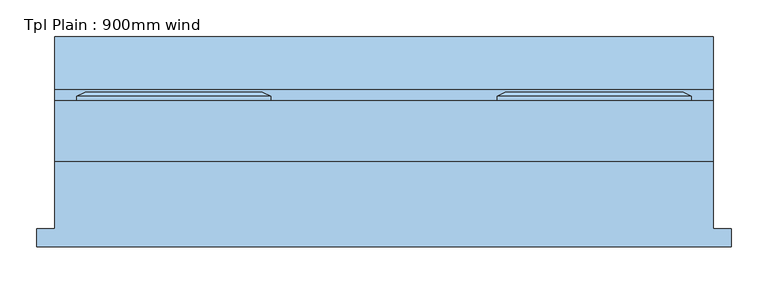
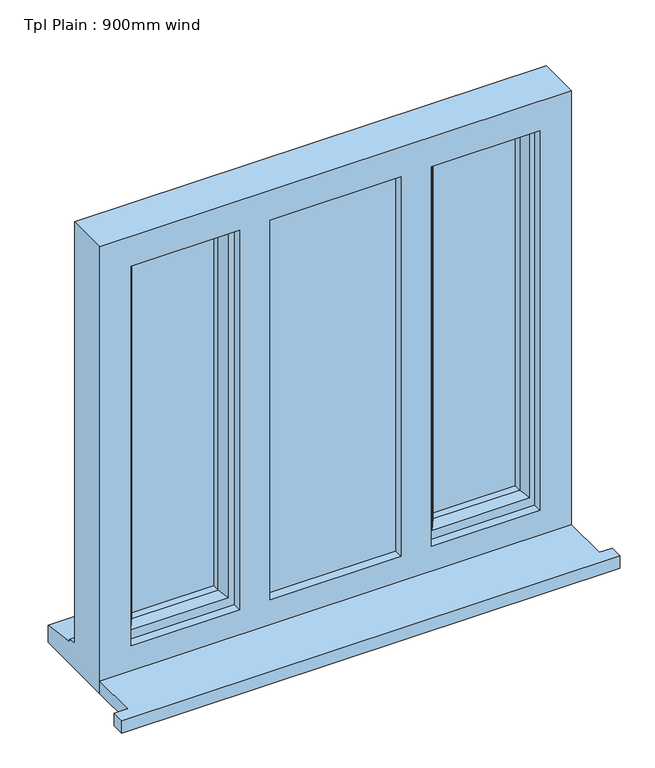
"""IFC4 building model written with IfcOpenShell, lengths in millimetres: window geometry, Tpl Plain : 900mm wind."""

from ifc_helpers import new_model, si_unit, frame, origin, place, context, project, spatial, polyline, outline, extrude, faceted_brep, source, transform, mapped, element, save


def tpl_plain_900mm_wind_8db11632(model_context):
    return source(origin(), model_context, "Body", "SolidModel", [
        extrude(outline(polyline([(-900.0, -129.0434322), (-900.0, -104.0434322), (-875.0, -104.0434322), (-875.0, -12.0434322), (25.0, -12.0434322), (25.0, -104.0434322), (50.0, -104.0434322), (50.0, -129.0434322), (-900.0, -129.0434322)])), frame((0.0, 0.0, 1500.0), z_axis=(0.0, 0.0, 1.0), x_axis=(1.0, 0.0, 0.0)), (0.0, 0.0, 1.0), 25.0),
        faceted_brep([(-270.0, 70.9565678, 2370.0), (-270.0, 76.7300705, 2370.0), (-270.0, 76.7300705, 1553.0), (-270.0, 70.9565678, 1553.0), (-260.0, 5.9565678, 2360.0), (-260.0, 70.9565678, 2360.0), (-260.0, 70.9565678, 1563.0), (-260.0, 5.9565678, 1563.0), (-220.0, 20.4494677, 2320.0), (-230.1480377, 5.9565678, 2330.1480377), (-230.1480377, 5.9565678, 1592.8519623), (-220.0, 20.4494677, 1603.0), (-220.0, 34.9565678, 2320.0), (-220.0, 34.9565678, 1603.0), (-230.0, 58.9565678, 2330.0), (-230.0, 34.9565678, 2330.0), (-230.0, 34.9565678, 1593.0), (-230.0, 58.9565678, 1593.0), (-220.0, 76.7300705, 2320.0), (-220.0, 58.9565678, 2320.0), (-220.0, 58.9565678, 1603.0), (-220.0, 76.7300705, 1603.0), (-237.4457548, 82.5035732, 2337.4457548), (-237.4457548, 82.5035732, 1585.5542452), (-259.2153903, 82.5035732, 2359.2153903), (-259.2153903, 82.5035732, 1563.7846097), (-5.0, 76.7300705, 1553.0), (-5.0, 70.9565678, 1553.0), (-15.0, 70.9565678, 1563.0), (-15.0, 5.9565678, 1563.0), (-44.8519623, 5.9565678, 1592.8519623), (-55.0, 20.4494677, 1603.0), (-55.0, 34.9565678, 1603.0), (-45.0, 34.9565678, 1593.0), (-45.0, 58.9565678, 1593.0), (-55.0, 58.9565678, 1603.0), (-55.0, 76.7300705, 1603.0), (-37.5542452, 82.5035732, 1585.5542452), (-15.7846097, 82.5035732, 1563.7846097), (-5.0, 76.7300705, 2370.0), (-5.0, 70.9565678, 2370.0), (-15.0, 70.9565678, 2360.0), (-15.0, 5.9565678, 2360.0), (-44.8519623, 5.9565678, 2330.1480377), (-55.0, 20.4494677, 2320.0), (-55.0, 34.9565678, 2320.0), (-45.0, 34.9565678, 2330.0), (-45.0, 58.9565678, 2330.0), (-55.0, 58.9565678, 2320.0), (-55.0, 76.7300705, 2320.0), (-37.5542452, 82.5035732, 2337.4457548), (-15.7846097, 82.5035732, 2359.2153903)], [[[0, 1, 2, 3]], [[4, 5, 6, 7]], [[8, 9, 10, 11]], [[12, 8, 11, 13]], [[14, 15, 16, 17]], [[18, 19, 20, 21]], [[22, 18, 21, 23]], [[1, 24, 25, 2]], [[3, 2, 26, 27]], [[7, 6, 28, 29]], [[11, 10, 30, 31]], [[13, 11, 31, 32]], [[17, 16, 33, 34]], [[21, 20, 35, 36]], [[23, 21, 36, 37]], [[2, 25, 38, 26]], [[27, 26, 39, 40]], [[29, 28, 41, 42]], [[31, 30, 43, 44]], [[32, 31, 44, 45]], [[34, 33, 46, 47]], [[36, 35, 48, 49]], [[37, 36, 49, 50]], [[26, 38, 51, 39]], [[40, 39, 1, 0]], [[3, 27, 40, 0], [5, 41, 28, 6]], [[42, 41, 5, 4]], [[7, 29, 42, 4], [9, 43, 30, 10]], [[44, 43, 9, 8]], [[45, 44, 8, 12]], [[15, 46, 33, 16], [13, 32, 45, 12]], [[47, 46, 15, 14]], [[17, 34, 47, 14], [19, 48, 35, 20]], [[49, 48, 19, 18]], [[50, 49, 18, 22]], [[24, 51, 38, 25], [23, 37, 50, 22]], [[39, 51, 24, 1]]]),
        faceted_brep([(-580.0, 70.9565678, 2370.0), (-580.0, 76.7300705, 2370.0), (-845.0, 76.7300705, 2370.0), (-845.0, 70.9565678, 2370.0), (-590.0, 5.9565678, 2360.0), (-590.0, 70.9565678, 2360.0), (-835.0, 70.9565678, 2360.0), (-835.0, 5.9565678, 2360.0), (-630.0, 20.4494677, 2320.0), (-619.8519623, 5.9565678, 2330.1480377), (-805.1480377, 5.9565678, 2330.1480377), (-795.0, 20.4494677, 2320.0), (-630.0, 34.9565678, 2320.0), (-795.0, 34.9565678, 2320.0), (-620.0, 58.9565678, 2330.0), (-620.0, 34.9565678, 2330.0), (-805.0, 34.9565678, 2330.0), (-805.0, 58.9565678, 2330.0), (-630.0, 76.7300705, 2320.0), (-630.0, 58.9565678, 2320.0), (-795.0, 58.9565678, 2320.0), (-795.0, 76.7300705, 2320.0), (-611.1854344, 82.5035732, 2338.8145656), (-813.8145656, 82.5035732, 2338.8145656), (-591.6307806, 82.5035732, 2358.3692194), (-833.3692194, 82.5035732, 2358.3692194), (-845.0, 76.7300705, 1553.0), (-845.0, 70.9565678, 1553.0), (-835.0, 70.9565678, 1563.0), (-835.0, 5.9565678, 1563.0), (-805.1480377, 5.9565678, 1592.8519623), (-795.0, 20.4494677, 1603.0), (-795.0, 34.9565678, 1603.0), (-805.0, 34.9565678, 1593.0), (-805.0, 58.9565678, 1593.0), (-795.0, 58.9565678, 1603.0), (-795.0, 76.7300705, 1603.0), (-813.8145656, 82.5035732, 1584.1854344), (-833.3692194, 82.5035732, 1564.6307806), (-580.0, 76.7300705, 1553.0), (-580.0, 70.9565678, 1553.0), (-590.0, 70.9565678, 1563.0), (-590.0, 5.9565678, 1563.0), (-619.8519623, 5.9565678, 1592.8519623), (-630.0, 20.4494677, 1603.0), (-630.0, 34.9565678, 1603.0), (-620.0, 34.9565678, 1593.0), (-620.0, 58.9565678, 1593.0), (-630.0, 58.9565678, 1603.0), (-630.0, 76.7300705, 1603.0), (-611.1854344, 82.5035732, 1584.1854344), (-591.6307806, 82.5035732, 1564.6307806)], [[[0, 1, 2, 3]], [[4, 5, 6, 7]], [[8, 9, 10, 11]], [[12, 8, 11, 13]], [[14, 15, 16, 17]], [[18, 19, 20, 21]], [[22, 18, 21, 23]], [[1, 24, 25, 2]], [[3, 2, 26, 27]], [[7, 6, 28, 29]], [[11, 10, 30, 31]], [[13, 11, 31, 32]], [[17, 16, 33, 34]], [[21, 20, 35, 36]], [[23, 21, 36, 37]], [[2, 25, 38, 26]], [[27, 26, 39, 40]], [[0, 3, 27, 40], [41, 28, 6, 5]], [[29, 28, 41, 42]], [[4, 7, 29, 42], [43, 30, 10, 9]], [[31, 30, 43, 44]], [[32, 31, 44, 45]], [[46, 33, 16, 15], [12, 13, 32, 45]], [[34, 33, 46, 47]], [[14, 17, 34, 47], [48, 35, 20, 19]], [[36, 35, 48, 49]], [[37, 36, 49, 50]], [[51, 38, 25, 24], [22, 23, 37, 50]], [[26, 38, 51, 39]], [[40, 39, 1, 0]], [[42, 41, 5, 4]], [[44, 43, 9, 8]], [[45, 44, 8, 12]], [[47, 46, 15, 14]], [[49, 48, 19, 18]], [[50, 49, 18, 22]], [[39, 51, 24, 1]]]),
        faceted_brep([(25.0, -12.0434322, 2400.0), (-875.0, -12.0434322, 2400.0), (-875.0, -12.0434322, 1500.0), (25.0, -12.0434322, 1500.0), (-35.0, -12.0434322, 2340.0), (-35.0, -12.0434322, 1575.0), (-242.0, -12.0434322, 1575.0), (-242.0, -12.0434322, 2340.0), (-300.0, -12.0434322, 2340.0), (-300.0, -12.0434322, 1575.0), (-550.0, -12.0434322, 1575.0), (-550.0, -12.0434322, 2340.0), (-608.0, -12.0434322, 2340.0), (-608.0, -12.0434322, 1575.0), (-815.0, -12.0434322, 1575.0), (-815.0, -12.0434322, 2340.0), (-875.0, 70.9565678, 2400.0), (-875.0, 70.9565678, 1551.0), (-875.0, 85.9565678, 1549.68767), (-875.0, 85.9565678, 1544.7449676), (-875.0, 158.4565678, 1533.8088847), (-875.0, 158.4565678, 1500.0), (25.0, 70.9565678, 2400.0), (25.0, 70.9565678, 1551.0), (-835.0, 70.9565678, 2360.0), (-835.0, 70.9565678, 1563.0), (-590.0, 70.9565678, 1563.0), (-590.0, 70.9565678, 2360.0), (-550.0, 70.9565678, 2360.0), (-550.0, 70.9565678, 1563.0), (-300.0, 70.9565678, 1563.0), (-300.0, 70.9565678, 2360.0), (-260.0, 70.9565678, 2360.0), (-260.0, 70.9565678, 1563.0), (-15.0, 70.9565678, 1563.0), (-15.0, 70.9565678, 2360.0), (-835.0, 5.9565678, 2360.0), (-835.0, 5.9565678, 1563.0), (-560.0, 5.9565678, 2360.0), (-290.0, 5.9565678, 2360.0), (-290.0, 5.9565678, 1563.0), (-560.0, 5.9565678, 1563.0), (-300.0, 5.9565678, 2340.0), (-550.0, 5.9565678, 2340.0), (-550.0, 5.9565678, 1575.0), (-300.0, 5.9565678, 1575.0), (-260.0, 5.9565678, 2360.0), (-15.0, 5.9565678, 2360.0), (-15.0, 5.9565678, 1563.0), (-260.0, 5.9565678, 1563.0), (-35.0, 5.9565678, 2340.0), (-242.0, 5.9565678, 2340.0), (-242.0, 5.9565678, 1575.0), (-35.0, 5.9565678, 1575.0), (-590.0, 5.9565678, 2360.0), (-590.0, 5.9565678, 1563.0), (-608.0, 5.9565678, 2340.0), (-815.0, 5.9565678, 2340.0), (-815.0, 5.9565678, 1575.0), (-608.0, 5.9565678, 1575.0), (-550.0, 29.9565678, 2360.0), (-300.0, 29.9565678, 2360.0), (-290.0, 29.9565678, 2360.0), (-560.0, 29.9565678, 2360.0), (25.0, 158.4565678, 1500.0), (25.0, 158.4565678, 1533.8088847), (25.0, 85.9565678, 1544.7449676), (25.0, 85.9565678, 1549.68767), (-550.0, 29.9565678, 1563.0), (-560.0, 29.9565678, 1563.0), (-290.0, 29.9565678, 1563.0), (-300.0, 29.9565678, 1563.0)], [[[0, 1, 2, 3], [4, 5, 6, 7], [8, 9, 10, 11], [12, 13, 14, 15]], [[2, 1, 16, 17, 18, 19, 20, 21]], [[17, 16, 22, 23], [24, 25, 26, 27], [28, 29, 30, 31], [32, 33, 34, 35]], [[25, 24, 36, 37]], [[38, 39, 40, 41], [42, 43, 44, 45]], [[46, 47, 48, 49], [50, 51, 52, 53]], [[36, 54, 55, 37], [56, 57, 58, 59]], [[57, 15, 14, 58]], [[1, 0, 22, 16]], [[36, 24, 27, 54]], [[35, 47, 46, 32]], [[60, 28, 31, 61, 62, 39, 38, 63]], [[15, 57, 56, 12]], [[50, 4, 7, 51]], [[11, 43, 42, 8]], [[23, 22, 0, 3, 64, 65, 66, 67]], [[35, 34, 48, 47]], [[4, 50, 53, 5]], [[43, 11, 10, 44]], [[12, 56, 59, 13]], [[27, 26, 55, 54]], [[29, 28, 60, 68]], [[68, 60, 63, 69]], [[69, 63, 38, 41]], [[62, 70, 40, 39]], [[70, 62, 61, 71]], [[71, 61, 31, 30]], [[33, 32, 46, 49]], [[51, 7, 6, 52]], [[8, 42, 45, 9]], [[64, 3, 2, 21]], [[65, 64, 21, 20]], [[66, 65, 20, 19]], [[67, 66, 19, 18]], [[23, 67, 18, 17]], [[26, 25, 37, 55]], [[34, 33, 49, 48]], [[41, 40, 70, 71, 30, 29, 68, 69]], [[6, 5, 53, 52]], [[45, 44, 10, 9]], [[59, 58, 14, 13]]]),
        extrude(outline(polyline([(-620.0, 34.9565678), (-805.0, 34.9565678), (-805.0, 58.9565678), (-620.0, 58.9565678), (-620.0, 34.9565678)])), frame((0.0, 0.0, 1593.0), z_axis=(0.0, 0.0, 1.0), x_axis=(1.0, 0.0, 0.0)), (0.0, 0.0, 1.0), 737.0),
        extrude(outline(polyline([(-560.0, 29.9565678), (-290.0, 29.9565678), (-290.0, 5.9565678), (-560.0, 5.9565678), (-560.0, 29.9565678)])), frame((0.0, 0.0, 1563.0), z_axis=(0.0, 0.0, 1.0), x_axis=(1.0, 0.0, 0.0)), (0.0, 0.0, 1.0), 797.0),
        extrude(outline(polyline([(-45.0, 34.9565678), (-230.0, 34.9565678), (-230.0, 58.9565678), (-45.0, 58.9565678), (-45.0, 34.9565678)])), frame((0.0, 0.0, 1593.0), z_axis=(0.0, 0.0, 1.0), x_axis=(1.0, 0.0, 0.0)), (0.0, 0.0, 1.0), 737.0),
    ])


if __name__ == "__main__":
    model = new_model("IFC4")
    model_context = context("Model", 3, world=origin())
    ifc_project = project(units=[si_unit("LENGTHUNIT", "METRE", prefix="MILLI")], contexts=[model_context])
    site = spatial("IfcSite", under=ifc_project)
    building = spatial("IfcBuilding", under=site)
    placement = place(None, origin())
    tpl_plain_900mm_wind_shape = tpl_plain_900mm_wind_8db11632(model_context)
    element("IfcWindow", 1, ObjectType="Tpl Plain : 900mm wind", at=placement, inside=building, context=model_context, shape_type="MappedRepresentation", body=[
        mapped(tpl_plain_900mm_wind_shape, transform((0.0, 0.0, 0.0), x_axis=(1.0, 0.0, 0.0), y_axis=(0.0, 1.0, 0.0), z_axis=(0.0, 0.0, 1.0))),
    ])
    save(model, "model.ifc")

# Revit data of these elements
# Type "Tpl Plain : 900mm wind"
#   Type Mark = "35"
#   Operation = "TriplePanelVertical"
#   Manufacturer = "Revit"
#   Keynote = "L10"
#   Analytic Construction = "<None>"
#   Wrap Layers (Ext) from Ext = 102.5 mm
#   Wrap Layers (Int) from Ext = 177.5 mm
#   Window Board Projection = 25 mm
#   Window Board Extension = 25 mm
#   Rough Width = 900 mm
#   Rough Height = 900 mm
#   Height = 900 mm
#   Width = 900 mm
#   Glazing Thickness = 24 mm
#   FrameOffset - External = 50 mm
#   Frame Depth = 65 mm
#   Default Head Height = 2400 mm
#   Cill Depth = 87.5 mm
#   Cavity Closer Width = 50 mm
#   Cavity Closer Offset from Ext = 102.5 mm
#   Cavity Closer Depth = 85 mm
#   Vis - Cavity Closers = yes
#   Define Thermal Properties by = 1
#   Material Trim = Window Frame
#   Material Glass = Glass
#   Material Frame = Window Frame
#   Wall Closure = (empty or 0)
# Element 1 (IfcWindow, "Tpl Plain : 900mm wind")
#   Materials on its faces: "Window Frame", "Glass"
# Materials
#   "Window Frame": colour RGB 249 249 249, transparency 0, Keynote = "L10", Cost = 0
#   "Glass": class "Glass", colour RGB 0 128 192, transparency 0.9, Description = "Soda Lime Glass", Cost = 0
